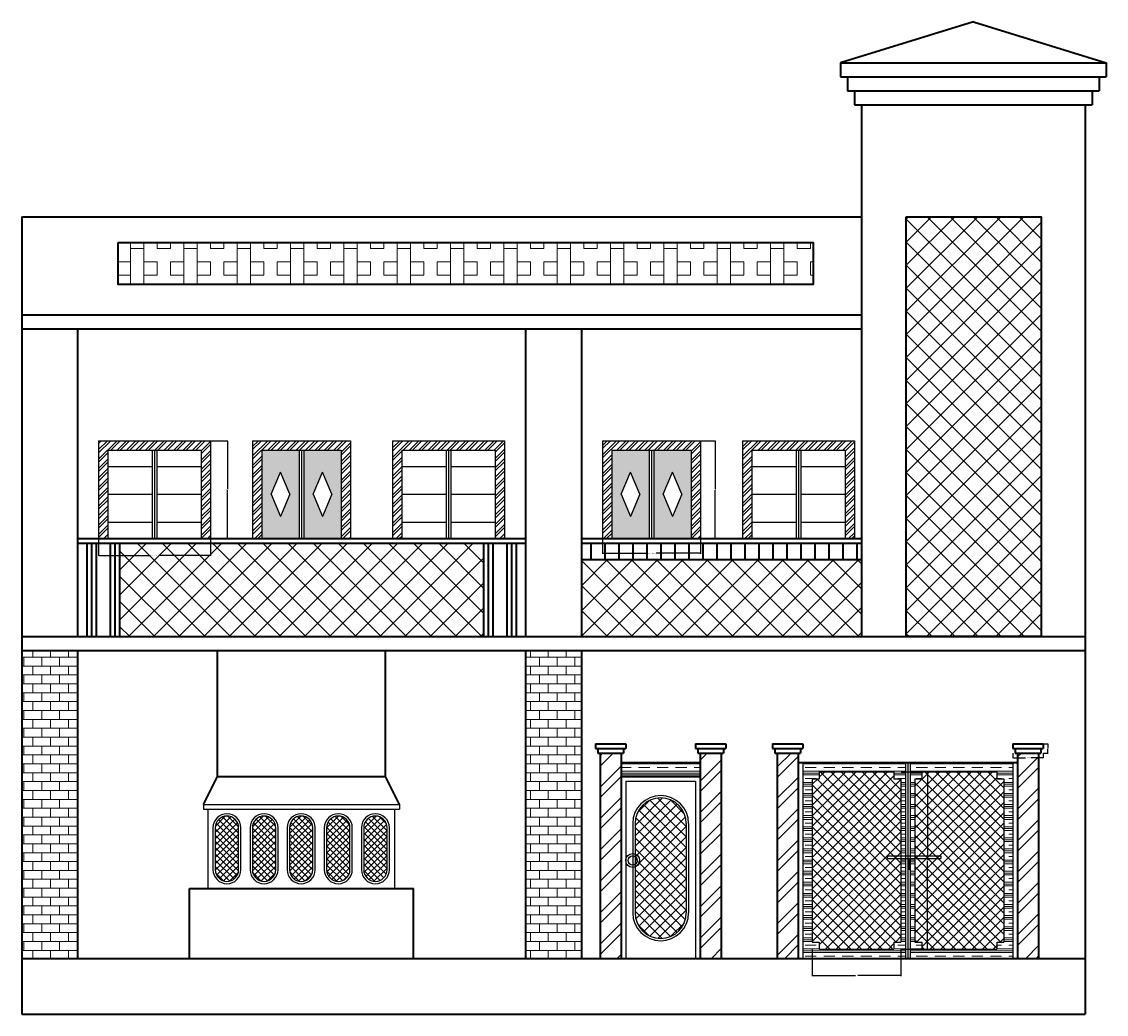
# Model space of a CAD drawing. Units: inches. Extents: x 1942 to 2407, y 597 to 1023.
import ezdxf

# ---------------------------------------------------------------- set-up
doc = ezdxf.new("R2010")
doc.units = ezdxf.units.IN
for name, color, linetype, lineweight in [('A-ANNO-DIMS', 2, 'Continuous', 18), ('A-DOOR', 3, 'Continuous', 25), ('A-DOOR-PATT', 252, 'Continuous', 13), ('A-ELEV', 7, 'Continuous', 35), ('A-GLAZ', 4, 'Continuous', 25), ('A-GLAZ-PATT', 252, 'Continuous', 13), ('A-WALL-PATT', 8, 'Continuous', 13)]:
    doc.layers.add(name, color=color, linetype=linetype, lineweight=lineweight)
doc.styles.get("Standard").update_dxf_attribs({"font": 'arial.ttf'})
doc.dimstyles.get("Standard").update_dxf_attribs({"dimtxt": 0.18, "dimasz": 0.18, "dimexe": 0.18, "dimexo": 0.0625, "dimgap": 0.09, "dimtad": 0, "dimtih": 1, "dimtoh": 1, "dimdec": 4, "dimzin": 0, "dimdsep": 46, "dimtxsty": 'Standard', "dimcen": 0.09, "dimadec": 0, "dimazin": 0, "dimtfac": 1, "dimtdec": 4, "dimtofl": 0, "dimtmove": 0, "dimatfit": 3, "dimfxl": 1, "dimtolj": 1, "dimtzin": 0, "dimarcsym": 0})

# ---------------------------------------------------------------- blocks, each defined once
blk = doc.blocks.new('WIN-CASEMENT')
for p, q in [((0, 42), (0, 0)), ((0, 42), (48, 42)), ((48, 42), (48, 0)), ((4, 38), (44, 38)), ((4, 38), (4, 0)), ((23, 38), (23, 0)), ((24, 38), (24, 0)), ((25, 38), (25, 0)), ((44, 38), (44, 0)), ((4, 31), (23, 31)), ((25, 31), (44, 31)), ((4, 19), (23, 19)), ((25, 19), (44, 19)), ((4, 7), (23, 7)), ((25, 7), (44, 7))]:
    blk.add_line(p, q)
blk = doc.blocks.new('DOOR-GLAZED-DBL')
for p, q in [((0, 42), (42, 42)), ((0, 42), (0, 0)), ((0, 42), (42, 42)), ((42, 42), (42, 0)), ((4, 38), (38, 38)), ((4, 38), (4, 0)), ((20, 38), (20, 0)), ((21, 38), (21, 0)), ((22, 38), (22, 0)), ((38, 38), (38, 0)), ((8, 19), (12, 28.5)), ((16, 19), (12, 28.5)), ((26, 19), (30, 28.5)), ((34, 19), (30, 28.5)), ((8, 19), (12, 9.5)), ((16, 19), (12, 9.5)), ((26, 19), (30, 9.5)), ((34, 19), (30, 9.5))]:
    blk.add_line(p, q)
blk = doc.blocks.new('PIER-CAP')
for p, q in [((0, 4), (0, 2)), ((0, 4), (13, 4)), ((0, 2), (13, 2)), ((1, 2), (1, 0)), ((1, 0), (12, 0)), ((12, 2), (12, 0)), ((13, 4), (13, 2))]:
    blk.add_line(p, q)
blk = doc.blocks.new('GATE-LEAF')
for p, q in [((3, 76), (35.03, 76)), ((3, 76), (3, 73)), ((35.03, 76), (35.03, 73)), ((0, 73), (0, 3)), ((0, 73), (3, 73)), ((35.03, 73), (38.03, 73)), ((38.03, 73), (38.03, 3)), ((0, 3), (3, 3)), ((3, 3), (3, 0)), ((3, 0), (35.03, 0)), ((35.03, 3), (35.03, 0)), ((35.03, 3), (38.03, 3))]:
    blk.add_line(p, q)
blk = doc.blocks.new('*D5')
at = {"layer": 'A-ANNO-DIMS', "color": 0, "lineweight": -2, "transparency": 16777216}
for p, q in [((2367.15, 709.37), (2367.15, 707.31)), ((2367.33, 707.49), (2372.51, 707.49)), ((2379.97, 707.49), (2374.8, 707.49)), ((2380.15, 709.37), (2380.15, 707.31))]:
    blk.add_line(p, q, dxfattribs=at)
at = {"layer": 'A-ANNO-DIMS', "color": 0, "transparency": 16777216}
for points in [[(2367.33, 707.52), (2367.33, 707.46), (2367.15, 707.49)], [(2379.97, 707.52), (2379.97, 707.46), (2380.15, 707.49)]]:
    blk.add_solid(points, dxfattribs=at)
at = {"layer": 'Defpoints', "color": 0, "transparency": 16777216}
for p in [(2367.15, 709.44), (2380.15, 709.44), (2380.15, 707.49)]:
    blk.add_point(p, dxfattribs=at)
at = {"layer": 'A-ANNO-DIMS', "color": 0, "transparency": 16777216, "insert": (2373.65, 707.49), "char_height": 0.18, "attachment_point": 5}
blk.add_mtext('\\A1;PIER CAP 13 TYP.', dxfattribs=at)
blk = doc.blocks.new('*D6')
at = {"layer": 'A-ANNO-DIMS', "color": 0, "lineweight": -2, "transparency": 16777216}
for p, q in [((2380.22, 713.44), (2382.28, 713.44)), ((2382.1, 713.26), (2382.1, 711.62)), ((2380.22, 709.44), (2382.28, 709.44)), ((2382.1, 709.62), (2382.1, 711.26))]:
    blk.add_line(p, q, dxfattribs=at)
at = {"layer": 'A-ANNO-DIMS', "color": 0, "transparency": 16777216}
for points in [[(2382.07, 713.26), (2382.13, 713.26), (2382.1, 713.44)], [(2382.07, 709.62), (2382.13, 709.62), (2382.1, 709.44)]]:
    blk.add_solid(points, dxfattribs=at)
at = {"layer": 'Defpoints', "color": 0, "transparency": 16777216}
for p in [(2380.15, 713.44), (2382.1, 713.44), (2380.15, 709.44)]:
    blk.add_point(p, dxfattribs=at)
at = {"layer": 'A-ANNO-DIMS', "color": 0, "transparency": 16777216, "insert": (2382.1, 711.44), "char_height": 0.18, "attachment_point": 5}
blk.add_mtext('\\A1;4 TYP.', dxfattribs=at)
blk = doc.blocks.new('*D7')
at = {"layer": 'A-ANNO-DIMS', "color": 0, "lineweight": -2, "transparency": 16777216}
for p, q in [((1975.15, 801.37), (1975.15, 794.06)), ((2023.15, 801.37), (2023.15, 794.06)), ((1975.33, 794.24), (1997.31, 794.24)), ((2022.97, 794.24), (2001, 794.24))]:
    blk.add_line(p, q, dxfattribs=at)
at = {"layer": 'A-ANNO-DIMS', "color": 0, "transparency": 16777216}
for points in [[(1975.33, 794.27), (1975.33, 794.21), (1975.15, 794.24)], [(2022.97, 794.27), (2022.97, 794.21), (2023.15, 794.24)]]:
    blk.add_solid(points, dxfattribs=at)
at = {"layer": 'Defpoints', "color": 0, "transparency": 16777216}
for p in [(1975.15, 801.44), (2023.15, 801.44), (2023.15, 794.24)]:
    blk.add_point(p, dxfattribs=at)
at = {"layer": 'A-ANNO-DIMS', "color": 0, "transparency": 16777216, "insert": (1999.15, 794.24), "char_height": 0.18, "attachment_point": 5}
blk.add_mtext('\\A1;CASEMENT WINDOW 48 TYP.', dxfattribs=at)
blk = doc.blocks.new('*D8')
at = {"layer": 'A-ANNO-DIMS', "color": 0, "lineweight": -2, "transparency": 16777216}
for p, q in [((2023.22, 843.44), (2030.53, 843.44)), ((2030.35, 843.26), (2030.35, 822.62)), ((2030.35, 801.62), (2030.35, 822.26)), ((2023.22, 801.44), (2030.53, 801.44))]:
    blk.add_line(p, q, dxfattribs=at)
at = {"layer": 'A-ANNO-DIMS', "color": 0, "transparency": 16777216}
for points in [[(2030.32, 843.26), (2030.38, 843.26), (2030.35, 843.44)], [(2030.32, 801.62), (2030.38, 801.62), (2030.35, 801.44)]]:
    blk.add_solid(points, dxfattribs=at)
at = {"layer": 'Defpoints', "color": 0, "transparency": 16777216}
for p in [(2023.15, 843.44), (2030.35, 843.44), (2023.15, 801.44)]:
    blk.add_point(p, dxfattribs=at)
at = {"layer": 'A-ANNO-DIMS', "color": 0, "transparency": 16777216, "insert": (2030.35, 822.44), "char_height": 0.18, "attachment_point": 5}
blk.add_mtext('\\A1;42 TYP.', dxfattribs=at)
blk = doc.blocks.new('*D9')
at = {"layer": 'A-ANNO-DIMS', "color": 0, "lineweight": -2, "transparency": 16777216}
for p, q in [((2191.15, 801.37), (2191.15, 794.96)), ((2233.15, 801.37), (2233.15, 794.96)), ((2191.33, 795.14), (2210.12, 795.14)), ((2232.97, 795.14), (2214.18, 795.14))]:
    blk.add_line(p, q, dxfattribs=at)
at = {"layer": 'A-ANNO-DIMS', "color": 0, "transparency": 16777216}
for points in [[(2191.33, 795.17), (2191.33, 795.11), (2191.15, 795.14)], [(2232.97, 795.17), (2232.97, 795.11), (2233.15, 795.14)]]:
    blk.add_solid(points, dxfattribs=at)
at = {"layer": 'Defpoints', "color": 0, "transparency": 16777216}
for p in [(2191.15, 801.44), (2233.15, 801.44), (2233.15, 795.14)]:
    blk.add_point(p, dxfattribs=at)
at = {"layer": 'A-ANNO-DIMS', "color": 0, "transparency": 16777216, "insert": (2212.15, 795.14), "char_height": 0.18, "attachment_point": 5}
blk.add_mtext('\\A1;GLAZED DOUBLE DOOR 42 TYP.', dxfattribs=at)
blk = doc.blocks.new('*D10')
at = {"layer": 'A-ANNO-DIMS', "color": 0, "lineweight": -2, "transparency": 16777216}
for p, q in [((2233.22, 843.44), (2239.63, 843.44)), ((2239.45, 843.26), (2239.45, 822.62)), ((2239.45, 801.62), (2239.45, 822.26)), ((2233.22, 801.44), (2239.63, 801.44))]:
    blk.add_line(p, q, dxfattribs=at)
at = {"layer": 'A-ANNO-DIMS', "color": 0, "transparency": 16777216}
for points in [[(2239.42, 843.26), (2239.48, 843.26), (2239.45, 843.44)], [(2239.42, 801.62), (2239.48, 801.62), (2239.45, 801.44)]]:
    blk.add_solid(points, dxfattribs=at)
at = {"layer": 'Defpoints', "color": 0, "transparency": 16777216}
for p in [(2233.15, 843.44), (2239.45, 843.44), (2233.15, 801.44)]:
    blk.add_point(p, dxfattribs=at)
at = {"layer": 'A-ANNO-DIMS', "color": 0, "transparency": 16777216, "insert": (2239.45, 822.44), "char_height": 0.18, "attachment_point": 5}
blk.add_mtext('\\A1;42 TYP.', dxfattribs=at)
blk = doc.blocks.new('*D11')
at = {"layer": 'A-ANNO-DIMS', "color": 0, "lineweight": -2, "transparency": 16777216}
for p, q in [((2319.19, 701.44), (2330.71, 701.44)), ((2330.53, 701.26), (2330.53, 663.62)), ((2330.53, 625.62), (2330.53, 663.25)), ((2319.19, 625.44), (2330.71, 625.44))]:
    blk.add_line(p, q, dxfattribs=at)
at = {"layer": 'A-ANNO-DIMS', "color": 0, "transparency": 16777216}
for points in [[(2330.5, 701.26), (2330.56, 701.26), (2330.53, 701.44)], [(2330.5, 625.62), (2330.56, 625.62), (2330.53, 625.44)]]:
    blk.add_solid(points, dxfattribs=at)
at = {"layer": 'Defpoints', "color": 0, "transparency": 16777216}
for p in [(2319.13, 701.44), (2330.53, 701.44), (2319.13, 625.44)]:
    blk.add_point(p, dxfattribs=at)
at = {"layer": 'A-ANNO-DIMS', "color": 0, "transparency": 16777216, "insert": (2330.53, 663.44), "char_height": 0.18, "attachment_point": 5}
blk.add_mtext('\\A1;GATE LEAF 76 TYP.', dxfattribs=at)
blk = doc.blocks.new('*D12')
at = {"layer": 'A-ANNO-DIMS', "color": 0, "lineweight": -2, "transparency": 16777216}
for p, q in [((2281.1, 625.37), (2281.1, 613.86)), ((2319.13, 625.37), (2319.13, 613.86)), ((2281.28, 614.04), (2299.59, 614.04)), ((2318.95, 614.04), (2300.64, 614.04))]:
    blk.add_line(p, q, dxfattribs=at)
at = {"layer": 'A-ANNO-DIMS', "color": 0, "transparency": 16777216}
for points in [[(2281.28, 614.07), (2281.28, 614.01), (2281.1, 614.04)], [(2318.95, 614.07), (2318.95, 614.01), (2319.13, 614.04)]]:
    blk.add_solid(points, dxfattribs=at)
at = {"layer": 'Defpoints', "color": 0, "transparency": 16777216}
for p in [(2281.1, 625.44), (2319.13, 625.44), (2319.13, 614.04)]:
    blk.add_point(p, dxfattribs=at)
at = {"layer": 'A-ANNO-DIMS', "color": 0, "transparency": 16777216, "insert": (2300.12, 614.04), "char_height": 0.18, "attachment_point": 5}
blk.add_mtext('\\A1;38 TYP.', dxfattribs=at)

msp = doc.modelspace()

# ---------------------------------------------------------------- hatches: boundary and pattern name
at = {"layer": 'A-DOOR-PATT'}
h = msp.add_hatch(dxfattribs=at)
h.set_pattern_fill('CLAY', color=256)
h.paths.add_polyline_path([(2233.1, 705.44), (2199.1, 705.44), (2199.1, 699.44), (2233.1, 699.44)])
h.paths.add_polyline_path([(2367.15, 705.44), (2323.13, 705.44), (2323.13, 665.39), (2325.13, 665.39), (2325.13, 698.44), (2328.13, 698.44), (2328.13, 701.44), (2360.15, 701.44), (2360.15, 698.44), (2363.15, 698.44), (2363.15, 628.44), (2360.15, 628.44), (2360.15, 625.44), (2328.13, 625.44), (2328.13, 628.44), (2325.13, 628.44), (2325.13, 664.22), (2323.13, 664.22), (2323.13, 621.44), (2367.15, 621.44)])
h.paths.add_polyline_path([(2321.13, 664.22), (2319.13, 664.22), (2319.13, 628.44), (2316.13, 628.44), (2316.13, 625.44), (2284.1, 625.44), (2284.1, 628.44), (2281.1, 628.44), (2281.1, 698.44), (2284.1, 698.44), (2284.1, 701.44), (2316.13, 701.44), (2316.13, 698.44), (2319.13, 698.44), (2319.13, 665.39), (2321.13, 665.39), (2321.13, 705.44), (2277.1, 705.44), (2277.1, 621.44), (2321.13, 621.44)])
h = msp.add_hatch(dxfattribs=at)
h.set_pattern_fill('ANSI37', color=256)
h.paths.add_polyline_path([(2319.13, 698.44), (2316.13, 698.44), (2316.13, 701.44), (2284.1, 701.44), (2284.1, 698.44), (2281.1, 698.44), (2281.1, 628.44), (2284.1, 628.44), (2284.1, 625.44), (2316.13, 625.44), (2316.13, 628.44), (2319.13, 628.44)])
h.paths.add_polyline_path([(2363.15, 698.44), (2360.15, 698.44), (2360.15, 701.44), (2328.13, 701.44), (2328.13, 698.44), (2325.13, 698.44), (2325.13, 628.44), (2328.13, 628.44), (2328.13, 625.44), (2360.15, 625.44), (2360.15, 628.44), (2363.15, 628.44)])
h = msp.add_hatch(dxfattribs=at)
h.set_pattern_fill('ANSI37', color=256)
h.paths.add_polyline_path([(2227.1, 679.25, 1), (2205.1, 679.25), (2205.1, 641, 1), (2227.1, 641)])
at = {"layer": 'A-GLAZ-PATT'}
h = msp.add_hatch(dxfattribs=at)
h.set_pattern_fill('ANSI32', color=256, scale=0.3)
h.paths.add_polyline_path([(2149.15, 843.44), (2101.15, 843.44), (2101.15, 801.44), (2105.15, 801.44), (2105.15, 839.44), (2145.15, 839.44), (2145.15, 801.44), (2149.15, 801.44)])
h.paths.add_polyline_path([(2083.15, 843.44), (2041.15, 843.44), (2041.15, 801.44), (2045.15, 801.44), (2045.15, 839.44), (2079.15, 839.44), (2079.15, 801.44), (2083.15, 801.44)])
h.paths.add_polyline_path([(2023.15, 843.44), (1975.15, 843.44), (1975.15, 801.44), (1979.15, 801.44), (1979.15, 839.44), (2019.15, 839.44), (2019.15, 801.44), (2023.15, 801.44)])
h.paths.add_polyline_path([(2233.15, 843.44), (2191.15, 843.44), (2191.15, 801.44), (2195.15, 801.44), (2195.15, 839.44), (2211.15, 839.44), (2229.15, 839.44), (2229.15, 801.44), (2233.15, 801.44)])
h.paths.add_polyline_path([(2299.15, 843.44), (2251.15, 843.44), (2251.15, 801.44), (2255.15, 801.44), (2255.15, 839.44), (2295.15, 839.44), (2295.15, 801.44), (2299.15, 801.44)])
h = msp.add_hatch(dxfattribs=at)
h.set_pattern_fill('ANGLE', color=256, scale=0.3)
h.set_pattern_definition([(0, (0, 0), (0, 2.0955), [1.524, -0.5715]), (90, (0, 0), (-2.0955, 1e-16), [1.524, -0.5715])])
h.paths.add_polyline_path([(2079.15, 839.44), (2063.15, 839.44), (2063.15, 801.44), (2079.15, 801.44)])
h.paths.add_polyline_path([(2067.15, 820.44), (2071.15, 829.94), (2075.15, 820.44), (2071.15, 810.94)], flags=16)
h.paths.add_polyline_path([(2061.15, 839.44), (2045.15, 839.44), (2045.15, 801.44), (2061.15, 801.44)])
h.paths.add_polyline_path([(2053.15, 810.94), (2049.15, 820.44), (2053.15, 829.94), (2057.15, 820.44)], flags=16)
h.paths.add_polyline_path([(2211.15, 839.44), (2195.15, 839.44), (2195.15, 801.44), (2211.15, 801.44)])
h.paths.add_polyline_path([(2203.15, 810.94), (2199.15, 820.44), (2203.15, 829.94), (2207.15, 820.44)], flags=16)
h.paths.add_polyline_path([(2229.15, 839.44), (2213.15, 839.44), (2213.15, 801.44), (2229.15, 801.44)])
h.paths.add_polyline_path([(2221.15, 810.94), (2217.15, 820.44), (2221.15, 829.94), (2225.15, 820.44)], flags=16)
h = msp.add_hatch(dxfattribs=at)
h.set_pattern_fill('ANSI37', color=256, scale=0.6)
h.paths.add_polyline_path([(2025.15, 659.44, 1), (2035.15, 659.44), (2035.15, 677.46, 1), (2025.15, 677.46)])
h.paths.add_polyline_path([(2041.06, 659.44, 1), (2051.06, 659.44), (2051.06, 677.46, 1), (2041.06, 677.46)])
h.paths.add_polyline_path([(2066.97, 677.46, 1), (2056.97, 677.46), (2056.97, 659.44, 1), (2066.97, 659.44)])
h.paths.add_polyline_path([(2082.89, 677.46, 1), (2072.89, 677.46), (2072.89, 659.44, 1), (2082.89, 659.44)])
h.paths.add_polyline_path([(2098.8, 677.46, 1), (2088.8, 677.46), (2088.8, 659.44, 1), (2098.8, 659.44)])
at = {"layer": 'A-WALL-PATT'}
h = msp.add_hatch(dxfattribs=at)
h.set_pattern_fill('ANSI37', color=256, scale=2.2)
h.paths.add_polyline_path([(2379.29, 939.44), (2321.39, 939.44), (2321.39, 759.44), (2379.29, 759.44)])
h = msp.add_hatch(dxfattribs=at)
h.set_pattern_fill('BOX', color=256, scale=0.9)
h.paths.add_polyline_path([(2281.48, 928.48), (1983.46, 928.48), (1983.46, 910.44), (2281.48, 910.44)])
h = msp.add_hatch(dxfattribs=at)
h.set_pattern_fill('ANSI37', color=256, scale=2.4)
h.paths.add_polyline_path([(2302.15, 792.44), (2182.15, 792.44), (2182.15, 759.44), (2302.15, 759.44)])
h.paths.add_polyline_path([(2140.15, 799.44), (1984.15, 799.44), (1984.15, 759.44), (2140.15, 759.44)])
h = msp.add_hatch(dxfattribs=at)
h.set_pattern_fill('BRICK', color=256, scale=0.6)
h.paths.add_polyline_path([(2182.15, 753.44), (2158.15, 753.44), (2158.15, 621.44), (2182.15, 621.44)])
h.paths.add_polyline_path([(1942.15, 621.44), (1966.15, 621.44), (1966.15, 753.44), (1942.15, 753.44)])
h = msp.add_hatch(dxfattribs=at)
h.set_pattern_fill('ANSI32', color=256)
h.paths.add_polyline_path([(2242.1, 709.44), (2233.1, 709.44), (2233.1, 621.44), (2242.1, 621.44)])
h.paths.add_polyline_path([(2199.1, 709.44), (2190.1, 709.44), (2190.1, 621.44), (2199.1, 621.44)])
h.paths.add_polyline_path([(2275.1, 709.44), (2266.1, 709.44), (2266.1, 621.44), (2275.1, 621.44)])
h.paths.add_polyline_path([(2378.15, 709.44), (2369.15, 709.44), (2369.15, 621.44), (2378.15, 621.44)])

# ---------------------------------------------------------------- linework, layer by layer
at = {"layer": 'A-DOOR'}
for p, q in [((2277.1, 705.44), (2277.1, 621.44)), ((2321.13, 705.44), (2321.13, 621.44)), ((2322.13, 705.44), (2322.13, 621.44)), ((2323.13, 705.44), (2323.13, 621.44)), ((2367.15, 705.44), (2367.15, 621.44)), ((2201.1, 697.44), (2201.1, 621.44)), ((2201.1, 697.44), (2231.1, 697.44)), ((2201.1, 697.44), (2201.1, 621.44)), ((2231.1, 697.44), (2231.1, 621.44)), ((2204.1, 679.25), (2204.1, 641)), ((2205.1, 679.25), (2205.1, 641)), ((2227.1, 679.25), (2227.1, 641)), ((2228.1, 679.25), (2228.1, 641)), ((2313.32, 664.22), (2313.32, 665.39)), ((2313.32, 665.39), (2336.2, 665.39)), ((2333.86, 666), (2333.86, 666)), ((2336.2, 665.39), (2336.2, 664.22)), ((2313.32, 664.22), (2320.79, 664.22)), ((2319.13, 664.22), (2322.15, 664.22)), ((2322.15, 664.22), (2322.15, 659.66)), ((2322.79, 659.66), (2322.79, 664.22)), ((2322.79, 664.22), (2336.2, 664.22)), ((2322.15, 659.66), (2322.79, 659.66))]:
    msp.add_line(p, q, dxfattribs=at)
for radius in [2.96, 1.96]:
    msp.add_circle((2204.1, 663.41), radius, dxfattribs=at)
for centre, radius, start, end in [((2216.1, 679.25), 12, 0, 180), ((2216.1, 679.25), 11, 0, 180), ((2216.1, 641), 12, 180, 0), ((2216.1, 641), 11, 180, 0)]:
    msp.add_arc(centre, radius, start, end, dxfattribs=at)
at = {"layer": 'A-ELEV'}
for p, q in [((2350.15, 1023.13), (2293.15, 1005.44)), ((2350.15, 1023.13), (2407.15, 1005.44)), ((2293.15, 1005.44), (2407.15, 1005.44)), ((2293.15, 1005.44), (2293.15, 999.44)), ((2407.15, 1005.44), (2407.15, 999.44)), ((2293.15, 999.44), (2296.15, 999.44)), ((2296.15, 999.44), (2407.15, 999.44)), ((2296.15, 999.44), (2296.15, 993.44)), ((2404.15, 999.44), (2404.15, 993.44)), ((2296.15, 993.44), (2404.15, 993.44)), ((2299.15, 993.44), (2299.15, 987.44)), ((2401.15, 993.44), (2401.15, 987.44)), ((2299.15, 987.44), (2401.15, 987.44)), ((2302.15, 987.44), (2302.15, 759.44)), ((2398.15, 987.44), (2398.15, 597.44)), ((1942.15, 939.44), (1942.15, 597.44)), ((1942.15, 939.44), (2302.15, 939.44)), ((1942.15, 897.44), (2302.15, 897.44)), ((1942.15, 891.44), (2302.15, 891.44)), ((1966.15, 891.44), (1966.15, 759.44)), ((2158.15, 891.44), (2158.15, 759.44)), ((2182.15, 891.44), (2182.15, 759.44)), ((1966.15, 801.44), (2158.15, 801.44)), ((2182.15, 801.44), (2302.15, 801.44)), ((1966.15, 799.44), (2158.15, 799.44)), ((1966.15, 799.44), (1966.15, 759.44)), ((1970.15, 799.44), (1970.15, 759.44)), ((1972.15, 799.44), (1972.15, 759.44)), ((1974.15, 799.44), (1974.15, 759.44)), ((1980.15, 799.44), (1980.15, 759.44)), ((1982.15, 799.44), (1982.15, 759.44)), ((1984.15, 799.44), (1984.15, 759.44)), ((2140.15, 799.44), (2140.15, 759.44)), ((2142.15, 799.44), (2142.15, 759.44)), ((2144.15, 799.44), (2144.15, 759.44)), ((2150.15, 799.44), (2150.15, 759.44)), ((2152.15, 799.44), (2152.15, 759.44)), ((2154.15, 799.44), (2154.15, 759.44)), ((2158.15, 799.44), (2158.15, 759.44)), ((2182.15, 799.44), (2302.15, 799.44)), ((2186.15, 799.44), (2186.15, 792.44)), ((2192.15, 799.44), (2192.15, 792.44)), ((2198.15, 799.44), (2198.15, 792.44)), ((2204.15, 799.44), (2204.15, 792.44)), ((2210.15, 799.44), (2210.15, 792.44)), ((2216.15, 799.44), (2216.15, 792.44)), ((2222.15, 799.44), (2222.15, 792.44)), ((2228.15, 799.44), (2228.15, 792.44)), ((2234.15, 799.44), (2234.15, 792.44)), ((2240.15, 799.44), (2240.15, 792.44)), ((2246.15, 799.44), (2246.15, 792.44)), ((2252.15, 799.44), (2252.15, 792.44)), ((2258.15, 799.44), (2258.15, 792.44)), ((2264.15, 799.44), (2264.15, 792.44)), ((2270.15, 799.44), (2270.15, 792.44)), ((2276.15, 799.44), (2276.15, 792.44)), ((2282.15, 799.44), (2282.15, 792.44)), ((2288.15, 799.44), (2288.15, 792.44)), ((2294.15, 799.44), (2294.15, 792.44)), ((2300.15, 799.44), (2300.15, 792.44)), ((2182.15, 792.44), (2302.15, 792.44)), ((1942.15, 759.44), (2398.15, 759.44)), ((1942.15, 753.44), (2398.15, 753.44)), ((1966.15, 753.44), (1966.15, 621.44)), ((2026.15, 699.44), (2026.15, 753.44)), ((2098.15, 699.44), (2098.15, 753.44)), ((2158.15, 753.44), (2158.15, 621.44)), ((2182.15, 753.44), (2182.15, 621.44)), ((2190.1, 713.44), (2199.1, 713.44)), ((2233.1, 713.44), (2242.1, 713.44)), ((2190.1, 709.44), (2190.1, 621.44)), ((2199.1, 709.44), (2199.1, 621.44)), ((2233.1, 711.44), (2242.1, 711.44)), ((2233.1, 709.44), (2233.1, 621.44)), ((2233.1, 709.44), (2242.1, 709.44)), ((2242.1, 709.44), (2242.1, 621.44)), ((2266.1, 709.44), (2266.1, 621.44)), ((2275.1, 709.44), (2275.1, 621.44)), ((2369.15, 709.44), (2369.15, 621.44)), ((2378.15, 709.44), (2378.15, 621.44)), ((2199.1, 705.44), (2233.1, 705.44)), ((2275.1, 705.44), (2369.15, 705.44)), ((2020.15, 687.44), (2026.15, 699.44)), ((2026.15, 699.44), (2098.15, 699.44)), ((2104.15, 687.44), (2098.15, 699.44)), ((2199.1, 699.44), (2233.1, 699.44)), ((2014.15, 621.44), (2014.15, 651.44)), ((2014.15, 651.44), (2110.15, 651.44)), ((2110.15, 621.44), (2110.15, 651.44)), ((1942.15, 621.44), (2398.15, 621.44)), ((1966.15, 621.44), (2158.15, 621.44)), ((1942.15, 597.44), (2398.15, 597.44))]:
    msp.add_line(p, q, dxfattribs=at)
for points in [[(2321.39, 939.44), (2379.29, 939.44), (2379.29, 759.44), (2321.39, 759.44)], [(1983.46, 928.48), (2281.48, 928.48), (2281.48, 910.44), (1983.46, 910.44)]]:
    msp.add_lwpolyline(points, close=True, dxfattribs=at)
at = {"layer": 'A-GLAZ'}
for p, q in [((2195.15, 839.44), (2211.15, 839.44)), ((2020.15, 687.44), (2104.15, 687.44)), ((2020.15, 687.44), (2020.15, 685.44)), ((2020.15, 685.44), (2104.15, 685.44)), ((2022.15, 651.44), (2022.15, 685.44)), ((2102.15, 651.44), (2102.15, 685.44)), ((2104.15, 687.44), (2104.15, 685.44)), ((2022.15, 677.46), (2022.15, 677.46))]:
    msp.add_line(p, q, dxfattribs=at)
for points in [[(2036.15, 659.44), (2036.15, 677.46, 1), (2024.15, 677.46), (2024.15, 659.44, 1)], [(2035.15, 659.44), (2035.15, 677.46, 1), (2025.15, 677.46), (2025.15, 659.44, 1)], [(2040.06, 659.44, 1), (2052.06, 659.44), (2052.06, 677.46, 1), (2040.06, 677.46)], [(2041.06, 659.44, 1), (2051.06, 659.44), (2051.06, 677.46, 1), (2041.06, 677.46)], [(2055.97, 659.44, 1), (2067.97, 659.44), (2067.97, 677.46, 1), (2055.97, 677.46)], [(2056.97, 659.44, 1), (2066.97, 659.44), (2066.97, 677.46, 1), (2056.97, 677.46)], [(2071.89, 659.44, 1), (2083.89, 659.44), (2083.89, 677.46, 1), (2071.89, 677.46)], [(2072.89, 659.44, 1), (2082.89, 659.44), (2082.89, 677.46, 1), (2072.89, 677.46)], [(2087.8, 659.44, 1), (2099.8, 659.44), (2099.8, 677.46, 1), (2087.8, 677.46)], [(2088.8, 659.44, 1), (2098.8, 659.44), (2098.8, 677.46, 1), (2088.8, 677.46)]]:
    msp.add_lwpolyline(points, format="xyb", close=True, dxfattribs=at)

# ---------------------------------------------------------------- block references
at = {"layer": 'A-DOOR'}
for p in [(2281.1, 625.44), (2325.13, 625.44)]:
    msp.add_blockref('GATE-LEAF', p, dxfattribs=at)
at = {"layer": 'A-ELEV'}
for p in [(2188.1, 709.44), (2231.1, 709.44), (2264.1, 709.44), (2367.15, 709.44)]:
    msp.add_blockref('PIER-CAP', p, dxfattribs=at)
at = {"layer": 'A-GLAZ'}
for name, p in [('WIN-CASEMENT', (1975.15, 801.44)), ('DOOR-GLAZED-DBL', (2041.15, 801.44)), ('WIN-CASEMENT', (2101.15, 801.44)), ('DOOR-GLAZED-DBL', (2191.15, 801.44)), ('WIN-CASEMENT', (2251.15, 801.44))]:
    msp.add_blockref(name, p, dxfattribs=at)

# ---------------------------------------------------------------- dimensions: what is measured, and where the dimension line sits
at = {"layer": 'A-ANNO-DIMS'}
for base, p1, p2, text, picture, middle in [((2030.35, 843.44), (2023.15, 801.44), (2023.15, 843.44), '<> TYP.', '*D8', (2030.35, 822.44)), ((2239.45, 843.44), (2233.15, 801.44), (2233.15, 843.44), '<> TYP.', '*D10', (2239.45, 822.44)), ((2382.1, 713.44), (2380.15, 709.44), (2380.15, 713.44), '<> TYP.', '*D6', (2382.1, 711.44)), ((2330.53, 701.44), (2319.13, 625.44), (2319.13, 701.44), 'GATE LEAF <> TYP.', '*D11', (2330.53, 663.44))]:
    dim = msp.add_linear_dim(base=base, p1=p1, p2=p2, angle=90, text=text, dimstyle='Standard', override={"dimdec": 0, "dimlfac": 1, "dimrnd": 0, "dimzin": 0, "dimdsep": 46, "dimlunit": 2}, dxfattribs=at)
    dim.commit()
    dim.dimension.update_dxf_attribs({"geometry": picture, "text_midpoint": middle})
for base, p1, p2, text, picture, middle in [((2023.15, 794.24), (1975.15, 801.44), (2023.15, 801.44), 'CASEMENT WINDOW <> TYP.', '*D7', (1999.15, 794.24)), ((2233.15, 795.14), (2191.15, 801.44), (2233.15, 801.44), 'GLAZED DOUBLE DOOR <> TYP.', '*D9', (2212.15, 795.14)), ((2380.15, 707.49), (2367.15, 709.44), (2380.15, 709.44), 'PIER CAP <> TYP.', '*D5', (2373.65, 707.49)), ((2319.13, 614.04), (2281.1, 625.44), (2319.13, 625.44), '<> TYP.', '*D12', (2300.12, 614.04))]:
    dim = msp.add_linear_dim(base=base, p1=p1, p2=p2, text=text, dimstyle='Standard', override={"dimdec": 0, "dimlfac": 1, "dimrnd": 0, "dimzin": 0, "dimdsep": 46, "dimlunit": 2}, dxfattribs=at)
    dim.commit()
    dim.dimension.update_dxf_attribs({"geometry": picture, "text_midpoint": middle})

doc.saveas('drawing.dxf')
